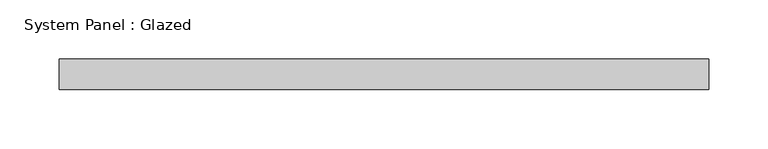
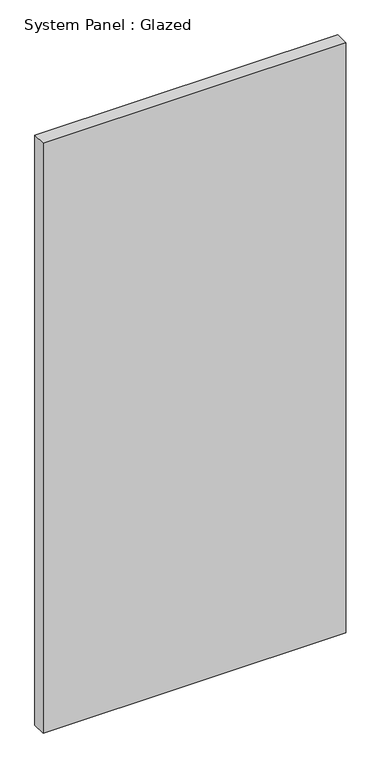
"""IFC4 building model written with IfcOpenShell, lengths in millimetres: plate geometry, System Panel : Glazed."""

from ifc_helpers import new_model, si_unit, origin, origin_with_axes, place, context, project, spatial, polyline, outline, extrude, source, transform, mapped, element, save


def system_panel_glazed_2d0a2ff2(model_context):
    return source(origin(), model_context, "Body", "SweptSolid", [
        extrude(outline(polyline([(273.05, 19.05), (-273.05, 19.05), (-273.05, 44.45), (273.05, 44.45), (273.05, 19.05)])), origin_with_axes(), (0.0, 0.0, 1.0), 1123.95),
    ])


if __name__ == "__main__":
    model = new_model("IFC4")
    model_context = context("Model", 3, world=origin())
    ifc_project = project(units=[si_unit("LENGTHUNIT", "METRE", prefix="MILLI")], contexts=[model_context])
    site = spatial("IfcSite", under=ifc_project)
    building = spatial("IfcBuilding", under=site)
    placement = place(None, origin())
    system_panel_glazed_shape = system_panel_glazed_2d0a2ff2(model_context)
    element("IfcPlate", 1, ObjectType="System Panel : Glazed", at=placement, inside=building, context=model_context, shape_type="MappedRepresentation", body=[
        mapped(system_panel_glazed_shape, transform((0.0, 0.0, 0.0), x_axis=(1.0, 0.0, 0.0), y_axis=(0.0, 1.0, 0.0), z_axis=(0.0, 0.0, 1.0))),
    ])
    save(model, "model.ifc")

# Revit data of these elements
# Type "System Panel : Glazed"
#   Construction Type Id = "GSP4R"
#   Analytic Construction = "1/8 in Pilkington single glazing"
#   Visual Light Transmittance = 0.9
#   Solar Heat Gain Coefficient = 0.86
#   Heat Transfer Coefficient (U) = 1.18115 BTU/(h·ft²·°F)
#   Define Thermal Properties by = 1
# Element 1 (IfcPlate, "System Panel : Glazed")
#   Materials on its faces: "Glass"
# Materials
#   "Glass": class "Glass", colour RGB 0 128 192, transparency 0.75, Description = "Soda Lime Glass", Cost = 0
